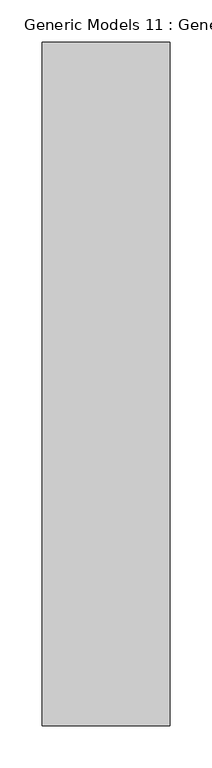
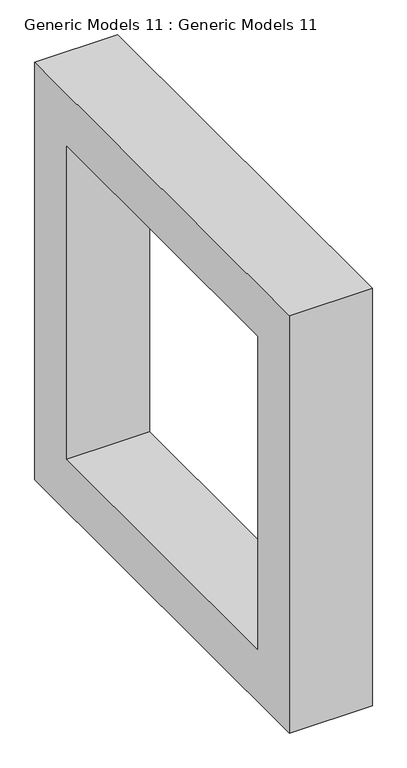
"""IFC4 building model written with IfcOpenShell, lengths in millimetres: proxy geometry, Generic Models 11 : Generic Models 11."""

from ifc_helpers import new_model, si_unit, frame, origin, place, context, project, spatial, polyline, outline, extrude, source, transform, mapped, element, save


def generic_models_11_generic_models_11_dfcfed8c(model_context):
    return source(origin(), model_context, "Body", "SweptSolid", [
        extrude(outline(polyline([(7048.5641252, 6291.5849297), (7861.3641252, 6291.5849297), (7861.3641252, 5478.7849297), (7048.5641252, 5478.7849297), (7048.5641252, 6291.5849297)]), holes=[polyline([(7150.1641252, 6189.9849297), (7150.1641252, 5580.3849297), (7759.7641252, 5580.3849297), (7759.7641252, 6189.9849297), (7150.1641252, 6189.9849297)])]), frame((-6249.7932997, 0.0, 0.0), z_axis=(1.0, 0.0, 0.0), x_axis=(0.0, 1.0, 0.0)), (0.0, 0.0, 1.0), 152.4),
    ])


if __name__ == "__main__":
    model = new_model("IFC4")
    model_context = context("Model", 3, world=origin())
    ifc_project = project(units=[si_unit("LENGTHUNIT", "METRE", prefix="MILLI")], contexts=[model_context])
    site = spatial("IfcSite", under=ifc_project)
    building = spatial("IfcBuilding", under=site)
    placement = place(None, origin())
    generic_models_11_generic_models_11_shape = generic_models_11_generic_models_11_dfcfed8c(model_context)
    element("IfcBuildingElementProxy", 1, Name="Generic Models 11 : Generic Models 11", ObjectType="Generic Models 11 : Generic Models 11", at=placement, inside=building, context=model_context, shape_type="MappedRepresentation", body=[
        mapped(generic_models_11_generic_models_11_shape, transform((0.0, 0.0, 0.0), x_axis=(1.0, 0.0, 0.0), y_axis=(0.0, 1.0, 0.0), z_axis=(0.0, 0.0, 1.0))),
    ])
    save(model, "model.ifc")

# Revit data of these elements
# Element 1 (IfcBuildingElementProxy, "Generic Models 11 : Generic Models 11")
#   Materials on its faces: "chocolate brown"
# Materials
#   "chocolate brown": class "Generic", colour RGB 120 120 120, transparency 0, Cost = 0
